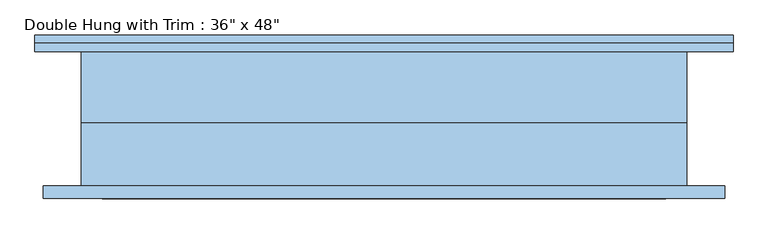
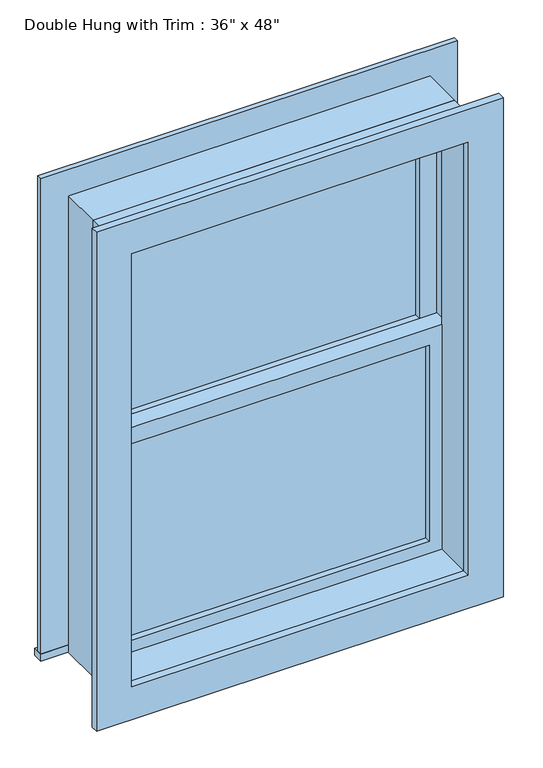
"""IFC4 building model written with IfcOpenShell, lengths in millimetres: window geometry."""

from ifc_helpers import new_model, si_unit, frame, origin, place, context, project, spatial, polyline, outline, extrude, source, transform, mapped, element, save


def window_1554aedb(model_context):
    return source(origin(), model_context, "Body", "SweptSolid", [
        extrude(outline(polyline([(-393.7, 22.225), (393.7, 22.225), (393.7, 9.525), (-393.7, 9.525), (-393.7, 22.225)])), frame((0.0, 0.0, 368.3), z_axis=(0.0, 0.0, 1.0), x_axis=(1.0, 0.0, 0.0)), (0.0, 0.0, 1.0), 523.875),
        extrude(outline(polyline([(936.625, -438.15), (323.85, -438.15), (323.85, 438.15), (936.625, 438.15), (936.625, -438.15)]), holes=[polyline([(892.175, -393.7), (892.175, 393.7), (368.3, 393.7), (368.3, -393.7), (892.175, -393.7)])]), frame((0.0, -6.35, 0.0), z_axis=(0.0, 1.0, 0.0), x_axis=(0.0, 0.0, 1.0)), (0.0, 0.0, 1.0), 44.45),
        extrude(outline(polyline([(-527.05, 127.0), (527.05, 127.0), (527.05, 101.6), (-527.05, 101.6), (-527.05, 127.0)])), frame((0.0, 0.0, 304.8), z_axis=(0.0, 0.0, 1.0), x_axis=(1.0, 0.0, 0.0)), (0.0, 0.0, 1.0), 19.05),
        extrude(outline(polyline([(1504.95, -438.15), (1504.95, 438.15), (323.85, 438.15), (323.85, 527.05), (1593.85, 527.05), (1593.85, -527.05), (323.85, -527.05), (323.85, -438.15), (1504.95, -438.15)])), frame((0.0, 101.6, 0.0), z_axis=(0.0, 1.0, 0.0), x_axis=(0.0, 0.0, 1.0)), (0.0, 0.0, 1.0), 12.7),
        extrude(outline(polyline([(1581.15, 514.35), (1581.15, -514.35), (247.65, -514.35), (247.65, 514.35), (1581.15, 514.35)]), holes=[polyline([(1492.25, 425.45), (336.55, 425.45), (336.55, -425.45), (1492.25, -425.45), (1492.25, 425.45)])]), frame((0.0, -120.65, 0.0), z_axis=(0.0, 1.0, 0.0), x_axis=(0.0, 0.0, 1.0)), (0.0, 0.0, 1.0), 19.05),
        extrude(outline(polyline([(393.7, 53.975), (-393.7, 53.975), (-393.7, 66.675), (393.7, 66.675), (393.7, 53.975)])), frame((0.0, 0.0, 936.625), z_axis=(0.0, 0.0, 1.0), x_axis=(1.0, 0.0, 0.0)), (0.0, 0.0, 1.0), 523.875),
        extrude(outline(polyline([(1504.95, -438.15), (892.175, -438.15), (892.175, 438.15), (1504.95, 438.15), (1504.95, -438.15)]), holes=[polyline([(1460.5, -393.7), (1460.5, 393.7), (936.625, 393.7), (936.625, -393.7), (1460.5, -393.7)])]), frame((0.0, 38.1, 0.0), z_axis=(0.0, 1.0, 0.0), x_axis=(0.0, 0.0, 1.0)), (0.0, 0.0, 1.0), 44.45),
        extrude(outline(polyline([(1524.0, -457.2), (304.8, -457.2), (304.8, 457.2), (1524.0, 457.2), (1524.0, -457.2)]), holes=[polyline([(1492.25, -425.45), (1492.25, 425.45), (336.55, 425.45), (336.55, -425.45), (1492.25, -425.45)])]), frame((0.0, -101.6, 0.0), z_axis=(0.0, 1.0, 0.0), x_axis=(0.0, 0.0, 1.0)), (0.0, 0.0, 1.0), 95.25),
        extrude(outline(polyline([(1524.0, 457.2), (1524.0, -457.2), (304.8, -457.2), (304.8, 457.2), (1524.0, 457.2)]), holes=[polyline([(1504.95, 438.15), (323.85, 438.15), (323.85, -438.15), (1504.95, -438.15), (1504.95, 438.15)])]), frame((0.0, -6.35, 0.0), z_axis=(0.0, 1.0, 0.0), x_axis=(0.0, 0.0, 1.0)), (0.0, 0.0, 1.0), 107.95),
    ])


if __name__ == "__main__":
    model = new_model("IFC4")
    model_context = context("Model", 3, world=origin())
    ifc_project = project(units=[si_unit("LENGTHUNIT", "METRE", prefix="MILLI")], contexts=[model_context])
    site = spatial("IfcSite", under=ifc_project)
    building = spatial("IfcBuilding", under=site)
    placement = place(None, origin())
    window_shape = window_1554aedb(model_context)
    element("IfcWindow", 1, ObjectType="Double Hung with Trim : 36\" x 48\"", at=placement, inside=building, context=model_context, shape_type="MappedRepresentation", body=[
        mapped(window_shape, transform((0.0, 0.0, 0.0), x_axis=(1.0, 0.0, 0.0), y_axis=(0.0, 1.0, 0.0), z_axis=(0.0, 0.0, 1.0))),
    ])
    save(model, "model.ifc")

# Revit data of these elements
# Type "Double Hung with Trim : 36\" x 48\""
#   Type Mark = "21"
#   Construction Type Id = "GSP4R"
#   Assembly Code = "B2020100"
#   Analytic Construction = "1/8 in Pilkington single glazing"
#   Visual Light Transmittance = 0.9
#   Solar Heat Gain Coefficient = 0.78
#   Heat Transfer Coefficient (U) = 0.6496 BTU/(h·ft²·°F)
#   Height = 4' - 0"
#   Default Sill Height = 1' - 0"
#   Trim Projection - Ext. = 0' - 0 1/2"
#   Trim Projection - Int. = 0' - 0 3/4"
#   Trim Width - Exterior = 0' - 3 1/2"
#   Trim Width - Interior = 0' - 3 1/2"
#   Width = 3' - 0"
#   Window Inset = 0' - 0 3/4"
#   Define Thermal Properties by = 1
#   Glass Pane Material = Glass
#   Sash Material = Sash
#   Trim Exterior Material = Trim
#   Trim Interior Material = Trim
#   Wall Closure = (empty or 0)
# Element 1 (IfcWindow, "Double Hung with Trim : 36\" x 48\"")
#   Materials on its faces: "Sash", "Trim", "Glass"
# Materials
#   "Glass": class "Glass", colour RGB 0 128 192, transparency 0.75, Description = "Soda Lime Glass", Cost = 0
#   "Sash": class "Wood", colour RGB 224 178 126, transparency 0
#   "Trim": class "Wood", colour RGB 224 178 126, transparency 0
